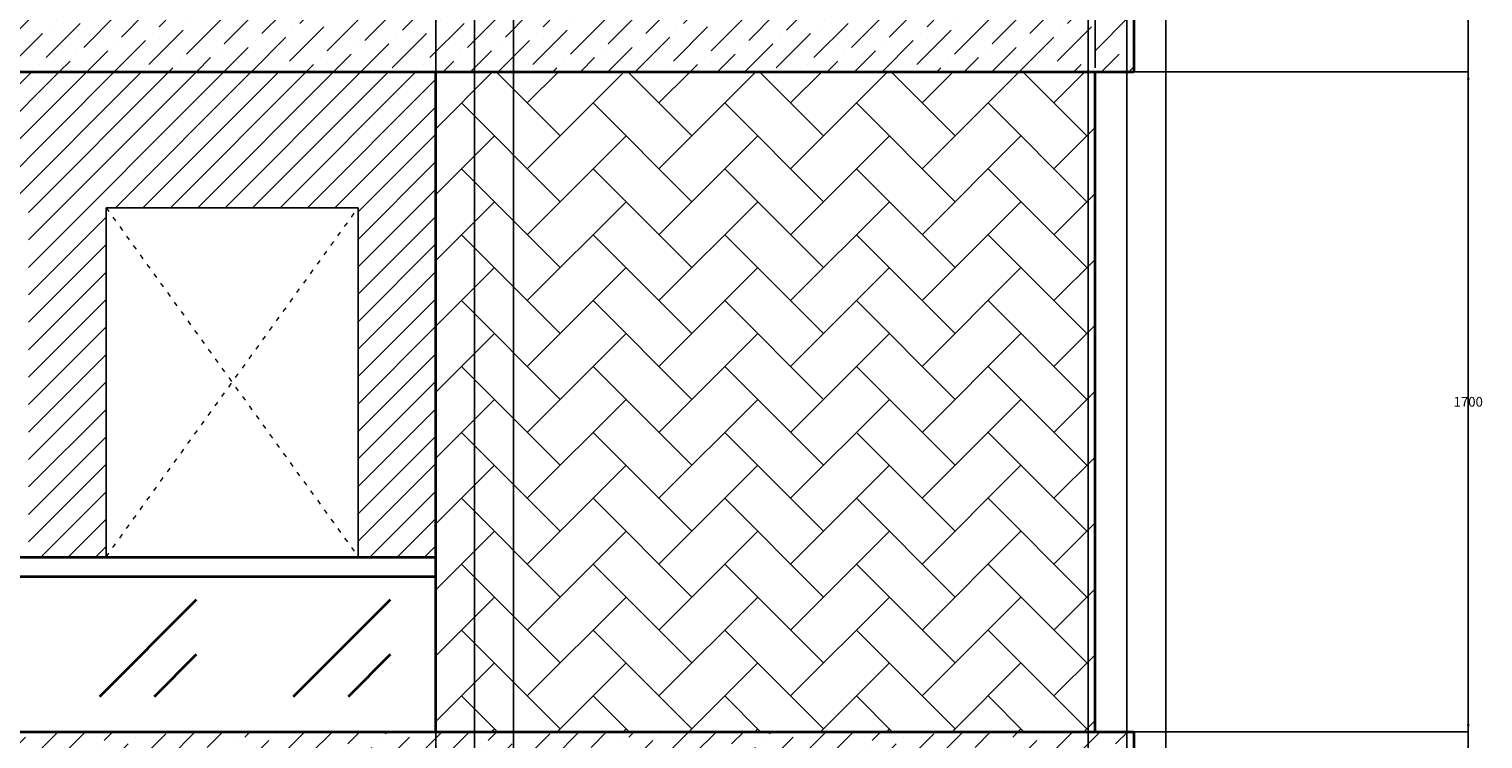
# Model space of a CAD drawing. Units: millimetres. Extents: x -692 to 9639, y -141 to 10345.
# Tile 18 of 19: x 5843 to 9592, y 4981 to 6809. Entities that reach past the tile are written whole.
import ezdxf

# ---------------------------------------------------------------- set-up
doc = ezdxf.new("R2010")
doc.units = ezdxf.units.MM
doc.header["$MEASUREMENT"] = 0
doc.linetypes.add('ACAD_ISO03W100', pattern=[30, 12, -18])
for name, color, linetype, lineweight in [('A-ANNO-DIMS', 2, 'Continuous', 18), ('A-DOOR', 3, 'Continuous', 25), ('A-DOOR-SWNG', 3, 'ACAD_ISO03W100', 18), ('A-ELEV', 7, 'Continuous', 35), ('A-ELEV-PATT', 8, 'Continuous', 13)]:
    doc.layers.add(name, color=color, linetype=linetype, lineweight=lineweight)
doc.styles.get("Standard").update_dxf_attribs({"font": 'arial.ttf'})
doc.dimstyles.get("Standard").update_dxf_attribs({"dimtxt": 25, "dimasz": 20, "dimexe": 0.18, "dimexo": 10, "dimgap": 10, "dimtad": 0, "dimtih": 1, "dimtoh": 1, "dimdec": 0, "dimzin": 0, "dimdsep": 46, "dimtxsty": 'Standard', "dimcen": 10, "dimadec": 0, "dimazin": 0, "dimtfac": 1, "dimtdec": 0, "dimtofl": 0, "dimtmove": 0, "dimatfit": 3, "dimfxl": 1, "dimtolj": 1, "dimtzin": 0, "dimarcsym": 0})

# ---------------------------------------------------------------- blocks, each defined once
blk = doc.blocks.new('*D7')
at = {"layer": 'A-ANNO-DIMS', "color": 0, "lineweight": -2, "transparency": 16777216}
for p, q in [((8481.5, 9848.8), (-649.1, 9848.8)), ((-648.9, 9828.8), (-648.9, 5124.9)), ((-648.9, 375.6), (-648.9, 5079.4)), ((2463.7, 355.6), (-649.1, 355.6))]:
    blk.add_line(p, q, dxfattribs=at)
at = {"layer": 'A-ANNO-DIMS', "color": 0, "lineweight": -3, "transparency": 16777216}
for points in [[(-652.2, 9828.8), (-645.6, 9828.8), (-648.9, 9848.8)], [(-652.2, 375.6), (-645.6, 375.6), (-648.9, 355.6)]]:
    blk.add_solid(points, dxfattribs=at)
at = {"layer": 'Defpoints', "color": 0, "lineweight": -3, "transparency": 16777216}
for p in [(-648.9, 9848.8), (8491.5, 9848.8), (2473.7, 355.6)]:
    blk.add_point(p, dxfattribs=at)
at = {"layer": 'A-ANNO-DIMS', "color": 0, "transparency": 16777216, "insert": (-648.9, 5102.2), "char_height": 25, "attachment_point": 5}
blk.add_mtext('\\A1;9493', dxfattribs=at)
blk = doc.blocks.new('*D9')
at = {"layer": 'A-ANNO-DIMS', "color": 0, "lineweight": -2, "transparency": 16777216}
for p, q in [((8501.5, 8848.8), (9553.9, 8848.8)), ((9553.7, 8828.8), (9553.7, 4874.9)), ((9553.7, 875.6), (9553.7, 4829.4)), ((9083.7, 855.6), (9553.9, 855.6))]:
    blk.add_line(p, q, dxfattribs=at)
at = {"layer": 'A-ANNO-DIMS', "color": 0, "lineweight": -3, "transparency": 16777216}
for points in [[(9550.4, 8828.8), (9557.1, 8828.8), (9553.7, 8848.8)], [(9550.4, 875.6), (9557.1, 875.6), (9553.7, 855.6)]]:
    blk.add_solid(points, dxfattribs=at)
at = {"layer": 'Defpoints', "color": 0, "lineweight": -3, "transparency": 16777216}
for p in [(8491.5, 8848.8), (9553.7, 8848.8), (9073.7, 855.6)]:
    blk.add_point(p, dxfattribs=at)
at = {"layer": 'A-ANNO-DIMS', "color": 0, "transparency": 16777216, "insert": (9553.7, 4852.2), "char_height": 25, "attachment_point": 5}
blk.add_mtext('\\A1;7993', dxfattribs=at)
blk = doc.blocks.new('*D32')
at = {"layer": 'A-ANNO-DIMS', "color": 0, "lineweight": -2, "transparency": 16777216}
for p, q in [((6871.7, 10328.8), (6851.7, 10328.8)), ((6891.7, 1865.6), (6891.7, 10329)), ((6991.7, 1765.6), (6991.7, 10329)), ((7011.7, 10328.8), (7031.7, 10328.8))]:
    blk.add_line(p, q, dxfattribs=at)
at = {"layer": 'A-ANNO-DIMS', "color": 0, "lineweight": -3, "transparency": 16777216}
for points in [[(6871.7, 10332.1), (6871.7, 10325.4), (6891.7, 10328.8)], [(7011.7, 10332.1), (7011.7, 10325.4), (6991.7, 10328.8)]]:
    blk.add_solid(points, dxfattribs=at)
at = {"layer": 'Defpoints', "color": 0, "lineweight": -3, "transparency": 16777216}
for p in [(6991.7, 10328.8), (6891.7, 1855.6), (6991.7, 1755.6)]:
    blk.add_point(p, dxfattribs=at)
at = {"layer": 'A-ANNO-DIMS', "color": 0, "transparency": 16777216, "insert": (6941.7, 10328.8), "char_height": 25, "attachment_point": 5}
blk.add_mtext('\\A1;100', dxfattribs=at)
blk = doc.blocks.new('*D33')
at = {"layer": 'A-ANNO-DIMS', "color": 0, "lineweight": -2, "transparency": 16777216}
for p, q in [((6971.7, 10328.8), (6951.7, 10328.8)), ((6991.7, 1765.6), (6991.7, 10329)), ((7091.7, 1665.6), (7091.7, 10329)), ((7111.7, 10328.8), (7131.7, 10328.8))]:
    blk.add_line(p, q, dxfattribs=at)
at = {"layer": 'A-ANNO-DIMS', "color": 0, "lineweight": -3, "transparency": 16777216}
for points in [[(6971.7, 10332.1), (6971.7, 10325.4), (6991.7, 10328.8)], [(7111.7, 10332.1), (7111.7, 10325.4), (7091.7, 10328.8)]]:
    blk.add_solid(points, dxfattribs=at)
at = {"layer": 'Defpoints', "color": 0, "lineweight": -3, "transparency": 16777216}
for p in [(7091.7, 10328.8), (6991.7, 1755.6), (7091.7, 1655.6)]:
    blk.add_point(p, dxfattribs=at)
at = {"layer": 'A-ANNO-DIMS', "color": 0, "transparency": 16777216, "insert": (7041.7, 10328.8), "char_height": 25, "attachment_point": 5}
blk.add_mtext('\\A1;100', dxfattribs=at)
blk = doc.blocks.new('*D34')
at = {"layer": 'A-ANNO-DIMS', "color": 0, "lineweight": -2, "transparency": 16777216}
for p, q in [((7091.7, 1665.6), (7091.7, 10329)), ((7111.7, 10328.8), (7786.7, 10328.8)), ((8553.7, 10328.8), (7878.8, 10328.8)), ((8573.7, 1665.6), (8573.7, 10329))]:
    blk.add_line(p, q, dxfattribs=at)
at = {"layer": 'A-ANNO-DIMS', "color": 0, "lineweight": -3, "transparency": 16777216}
for points in [[(7111.7, 10332.1), (7111.7, 10325.4), (7091.7, 10328.8)], [(8553.7, 10332.1), (8553.7, 10325.4), (8573.7, 10328.8)]]:
    blk.add_solid(points, dxfattribs=at)
at = {"layer": 'Defpoints', "color": 0, "lineweight": -3, "transparency": 16777216}
for p in [(8573.7, 10328.8), (7091.7, 1655.6), (8573.7, 1655.6)]:
    blk.add_point(p, dxfattribs=at)
at = {"layer": 'A-ANNO-DIMS', "color": 0, "transparency": 16777216, "insert": (7832.7, 10328.8), "char_height": 25, "attachment_point": 5}
blk.add_mtext('\\A1;1482', dxfattribs=at)
blk = doc.blocks.new('*D35')
at = {"layer": 'A-ANNO-DIMS', "color": 0, "lineweight": -2, "transparency": 16777216}
for p, q in [((8553.7, 10328.8), (8533.7, 10328.8)), ((8573.7, 1665.6), (8573.7, 10329)), ((8673.7, 1765.6), (8673.7, 10329)), ((8693.7, 10328.8), (8713.7, 10328.8))]:
    blk.add_line(p, q, dxfattribs=at)
at = {"layer": 'A-ANNO-DIMS', "color": 0, "lineweight": -3, "transparency": 16777216}
for points in [[(8553.7, 10332.1), (8553.7, 10325.4), (8573.7, 10328.8)], [(8693.7, 10332.1), (8693.7, 10325.4), (8673.7, 10328.8)]]:
    blk.add_solid(points, dxfattribs=at)
at = {"layer": 'Defpoints', "color": 0, "lineweight": -3, "transparency": 16777216}
for p in [(8673.7, 10328.8), (8673.7, 1755.6), (8573.7, 1655.6)]:
    blk.add_point(p, dxfattribs=at)
at = {"layer": 'A-ANNO-DIMS', "color": 0, "transparency": 16777216, "insert": (8623.7, 10328.8), "char_height": 25, "attachment_point": 5}
blk.add_mtext('\\A1;100', dxfattribs=at)
blk = doc.blocks.new('*D36')
at = {"layer": 'A-ANNO-DIMS', "color": 0, "lineweight": -2, "transparency": 16777216}
for p, q in [((8653.7, 10328.8), (8633.7, 10328.8)), ((8673.7, 1765.6), (8673.7, 10329)), ((8773.7, 1865.6), (8773.7, 10329)), ((8793.7, 10328.8), (8813.7, 10328.8))]:
    blk.add_line(p, q, dxfattribs=at)
at = {"layer": 'A-ANNO-DIMS', "color": 0, "lineweight": -3, "transparency": 16777216}
for points in [[(8653.7, 10332.1), (8653.7, 10325.4), (8673.7, 10328.8)], [(8793.7, 10332.1), (8793.7, 10325.4), (8773.7, 10328.8)]]:
    blk.add_solid(points, dxfattribs=at)
at = {"layer": 'Defpoints', "color": 0, "lineweight": -3, "transparency": 16777216}
for p in [(8773.7, 10328.8), (8773.7, 1855.6), (8673.7, 1755.6)]:
    blk.add_point(p, dxfattribs=at)
at = {"layer": 'A-ANNO-DIMS', "color": 0, "transparency": 16777216, "insert": (8723.7, 10328.8), "char_height": 25, "attachment_point": 5}
blk.add_mtext('\\A1;100', dxfattribs=at)
blk = doc.blocks.new('*D56')
at = {"layer": 'A-ANNO-DIMS', "color": 0, "lineweight": -2, "transparency": 16777216}
for p, q in [((5191.5, 6358.8), (5191.5, 10329)), ((5211.5, 10328.8), (5981.1, 10328.8)), ((6871.7, 10328.8), (6102.2, 10328.8)), ((6891.7, 6708.8), (6891.7, 10329))]:
    blk.add_line(p, q, dxfattribs=at)
at = {"layer": 'A-ANNO-DIMS', "color": 0, "lineweight": -3, "transparency": 16777216}
for points in [[(5211.5, 10332.1), (5211.5, 10325.4), (5191.5, 10328.8)], [(6871.7, 10332.1), (6871.7, 10325.4), (6891.7, 10328.8)]]:
    blk.add_solid(points, dxfattribs=at)
at = {"layer": 'Defpoints', "color": 0, "lineweight": -3, "transparency": 16777216}
for p in [(6891.7, 10328.8), (6891.7, 6698.8), (5191.5, 6348.8)]:
    blk.add_point(p, dxfattribs=at)
at = {"layer": 'A-ANNO-DIMS', "color": 0, "transparency": 16777216, "insert": (6041.6, 10328.8), "char_height": 25, "attachment_point": 5}
blk.add_mtext('\\A1;1700.2', dxfattribs=at)
blk = doc.blocks.new('*D57')
at = {"layer": 'A-ANNO-DIMS', "color": 0, "lineweight": -2, "transparency": 16777216}
for p, q in [((6891.7, 6708.8), (6891.7, 10329)), ((6911.7, 10328.8), (7680.9, 10328.8)), ((8571.5, 10328.8), (7802.4, 10328.8)), ((8591.5, 6708.8), (8591.5, 10329))]:
    blk.add_line(p, q, dxfattribs=at)
at = {"layer": 'A-ANNO-DIMS', "color": 0, "lineweight": -3, "transparency": 16777216}
for points in [[(6911.7, 10332.1), (6911.7, 10325.4), (6891.7, 10328.8)], [(8571.5, 10332.1), (8571.5, 10325.4), (8591.5, 10328.8)]]:
    blk.add_solid(points, dxfattribs=at)
at = {"layer": 'Defpoints', "color": 0, "lineweight": -3, "transparency": 16777216}
for p in [(8591.5, 10328.8), (6891.7, 6698.8), (8591.5, 6698.8)]:
    blk.add_point(p, dxfattribs=at)
at = {"layer": 'A-ANNO-DIMS', "color": 0, "transparency": 16777216, "insert": (7741.6, 10328.8), "char_height": 25, "attachment_point": 5}
blk.add_mtext('\\A1;1699.8', dxfattribs=at)
blk = doc.blocks.new('*D58')
at = {"layer": 'A-ANNO-DIMS', "color": 0, "lineweight": -2, "transparency": 16777216}
for p, q in [((8571.5, 10328.8), (8551.5, 10328.8)), ((8591.5, 6708.8), (8591.5, 10329)), ((8691.5, 6858.8), (8691.5, 10329)), ((8711.5, 10328.8), (8731.5, 10328.8))]:
    blk.add_line(p, q, dxfattribs=at)
at = {"layer": 'A-ANNO-DIMS', "color": 0, "lineweight": -3, "transparency": 16777216}
for points in [[(8571.5, 10332.1), (8571.5, 10325.4), (8591.5, 10328.8)], [(8711.5, 10332.1), (8711.5, 10325.4), (8691.5, 10328.8)]]:
    blk.add_solid(points, dxfattribs=at)
at = {"layer": 'Defpoints', "color": 0, "lineweight": -3, "transparency": 16777216}
for p in [(8691.5, 10328.8), (8691.5, 6848.8), (8591.5, 6698.8)]:
    blk.add_point(p, dxfattribs=at)
at = {"layer": 'A-ANNO-DIMS', "color": 0, "transparency": 16777216, "insert": (8641.5, 10328.8), "char_height": 25, "attachment_point": 5}
blk.add_mtext('\\A1;100', dxfattribs=at)
blk = doc.blocks.new('*D75')
at = {"layer": 'A-ANNO-DIMS', "color": 0, "lineweight": -2, "transparency": 16777216}
for p, q in [((8601.5, 6698.8), (9553.9, 6698.8)), ((9553.7, 6678.8), (9553.7, 5871.5)), ((9553.7, 5018.8), (9553.7, 5826)), ((8601.5, 4998.8), (9553.9, 4998.8))]:
    blk.add_line(p, q, dxfattribs=at)
at = {"layer": 'A-ANNO-DIMS', "color": 0, "lineweight": -3, "transparency": 16777216}
for points in [[(9550.4, 6678.8), (9557.1, 6678.8), (9553.7, 6698.8)], [(9550.4, 5018.8), (9557.1, 5018.8), (9553.7, 4998.8)]]:
    blk.add_solid(points, dxfattribs=at)
at = {"layer": 'Defpoints', "color": 0, "lineweight": -3, "transparency": 16777216}
for p in [(8591.5, 6698.8), (9553.7, 6698.8), (8591.5, 4998.8)]:
    blk.add_point(p, dxfattribs=at)
at = {"layer": 'A-ANNO-DIMS', "color": 0, "transparency": 16777216, "insert": (9553.7, 5848.8), "char_height": 25, "attachment_point": 5}
blk.add_mtext('\\A1;1700', dxfattribs=at)

msp = doc.modelspace()

# ---------------------------------------------------------------- hatches: boundary and pattern name
at = {"layer": 'A-ELEV-PATT'}
h = msp.add_hatch(dxfattribs=at)
h.set_pattern_fill('ANSI31', color=256, scale=400)
h.paths.add_polyline_path([(6891.746, 6698.772), (5191.547, 6698.772), (5191.547, 6348.772), (5841.547, 6348.772), (5841.547, 5448.772), (6041.547, 5448.772), (6041.547, 6348.772), (6691.547, 6348.772), (6691.547, 5448.772), (6891.746, 5448.772)])
h.paths.add_polyline_path([(5191.547, 6698.772), (3941.547, 6698.772), (3941.547, 5448.772), (4006.259, 5448.772), (4006.259, 6423.772), (5081.259, 6423.772), (5081.259, 5448.772), (5191.547, 5448.772), (5191.547, 6348.772)])
h.paths.add_polyline_path([(6891.746, 4848.772), (5191.547, 4848.772), (5191.547, 4497.772), (5841.746, 4497.772), (5841.746, 3598.27), (6041.746, 3598.27), (6041.746, 4497.772), (6691.746, 4497.772), (6691.746, 3598.27), (6891.746, 3598.27)])
h.paths.add_polyline_path([(6891.746, 8748.772), (5191.547, 8748.772), (5191.547, 8198.772), (5841.547, 8198.772), (5841.547, 7298.772), (6041.547, 7298.772), (6041.547, 8198.772), (6691.547, 8198.772), (6691.547, 7298.772), (6891.746, 7298.772)])
h = msp.add_hatch(dxfattribs=at)
h.set_pattern_fill('ANSI36', color=256, scale=400)
h.paths.add_polyline_path([(8691.547, 6848.772), (3791.547, 6848.772), (3791.547, 4848.772), (8691.547, 4848.772), (8691.547, 4998.772), (3941.547, 4998.772), (3941.547, 6698.772), (8691.547, 6698.772)])
h = msp.add_hatch(dxfattribs=at)
h.set_pattern_fill('AR-HBONE', color=256, scale=30)
h.paths.add_polyline_path([(8591.547, 6698.772), (6891.746, 6698.772), (6891.746, 4998.772), (8591.547, 4998.772)])

# ---------------------------------------------------------------- linework, layer by layer
at = {"layer": 'A-DOOR'}
for p, q in [((6041.547, 5448.772), (6041.547, 6348.772)), ((6041.547, 6348.772), (6691.547, 6348.772)), ((6691.547, 5448.772), (6691.547, 6348.772))]:
    msp.add_line(p, q, dxfattribs=at)
at = {"layer": 'A-DOOR-SWNG'}
for p, q in [((6041.547, 5449.27), (6691.746, 6348.772)), ((6041.547, 6348.772), (6691.746, 5449.27))]:
    msp.add_line(p, q, dxfattribs=at)
at = {"layer": 'A-ELEV'}
for p, q in [((8691.547, 6848.772), (8691.547, 6698.772)), ((3941.547, 6698.772), (8691.547, 6698.772)), ((6891.746, 4998.772), (6891.746, 6698.772)), ((8591.547, 4998.772), (8591.547, 6698.772)), ((3941.547, 5448.772), (6891.746, 5448.772)), ((3941.547, 5398.772), (6891.746, 5398.772)), ((6274.259, 5338.983), (6024.259, 5088.983)), ((6774.259, 5338.983), (6524.259, 5088.983)), ((6274.259, 5197.562), (6165.681, 5088.983)), ((6774.259, 5197.562), (6665.681, 5088.983)), ((3941.547, 4998.772), (8691.547, 4998.772)), ((8691.547, 4998.772), (8691.547, 4848.772))]:
    msp.add_line(p, q, dxfattribs=at)

# ---------------------------------------------------------------- dimensions: what is measured, and where the dimension line sits
at = {"layer": 'A-ANNO-DIMS'}
for base, p1, p2, override, picture, middle in [((6891.746, 10328.772), (5191.547, 6348.772), (6891.746, 6698.772), {"dimdec": 1, "dimlfac": 1, "dimrnd": 0, "dimzin": 0, "dimdsep": 46, "dimlunit": 2}, '*D56', (6041.646, 10328.772)), ((6991.746, 10328.772), (6891.746, 1855.575), (6991.746, 1755.575), {"dimdec": 0, "dimlfac": 1, "dimrnd": 0, "dimzin": 0, "dimdsep": 46, "dimlunit": 2}, '*D32', (6941.746, 10328.772)), ((8591.547, 10328.772), (6891.746, 6698.772), (8591.547, 6698.772), {"dimdec": 1, "dimlfac": 1, "dimrnd": 0, "dimzin": 0, "dimdsep": 46, "dimlunit": 2}, '*D57', (7741.646, 10328.772)), ((7091.746, 10328.772), (6991.746, 1755.575), (7091.746, 1655.575), {"dimdec": 0, "dimlfac": 1, "dimrnd": 0, "dimzin": 0, "dimdsep": 46, "dimlunit": 2}, '*D33', (7041.746, 10328.772)), ((8573.746, 10328.772), (7091.746, 1655.575), (8573.746, 1655.575), {"dimdec": 0, "dimlfac": 1, "dimrnd": 0, "dimzin": 0, "dimdsep": 46, "dimlunit": 2}, '*D34', (7832.746, 10328.772)), ((8673.746, 10328.772), (8573.746, 1655.575), (8673.746, 1755.575), {"dimdec": 0, "dimlfac": 1, "dimrnd": 0, "dimzin": 0, "dimdsep": 46, "dimlunit": 2}, '*D35', (8623.746, 10328.772)), ((8691.547, 10328.772), (8591.547, 6698.772), (8691.547, 6848.772), {"dimdec": 0, "dimlfac": 1, "dimrnd": 0, "dimzin": 0, "dimdsep": 46, "dimlunit": 2}, '*D58', (8641.547, 10328.772)), ((8773.746, 10328.772), (8673.746, 1755.575), (8773.746, 1855.575), {"dimdec": 0, "dimlfac": 1, "dimrnd": 0, "dimzin": 0, "dimdsep": 46, "dimlunit": 2}, '*D36', (8723.746, 10328.772))]:
    dim = msp.add_linear_dim(base=base, p1=p1, p2=p2, dimstyle='Standard', override=override, dxfattribs=at)
    dim.commit()
    dim.dimension.update_dxf_attribs({"geometry": picture, "text_midpoint": middle})
for base, p1, p2, picture, middle in [((-648.912, 9848.772), (2473.746, 355.575), (8491.547, 9848.772), '*D7', (-648.912, 5102.173)), ((9553.746, 8848.772), (9073.746, 855.575), (8491.547, 8848.772), '*D9', (9553.746, 4852.173)), ((9553.746, 6698.772), (8591.547, 4998.772), (8591.547, 6698.772), '*D75', (9553.746, 5848.772))]:
    dim = msp.add_linear_dim(base=base, p1=p1, p2=p2, angle=90, dimstyle='Standard', override={"dimdec": 0, "dimlfac": 1, "dimrnd": 0, "dimzin": 0, "dimdsep": 46, "dimlunit": 2}, dxfattribs=at)
    dim.commit()
    dim.dimension.update_dxf_attribs({"geometry": picture, "text_midpoint": middle})

doc.saveas('drawing.dxf')
